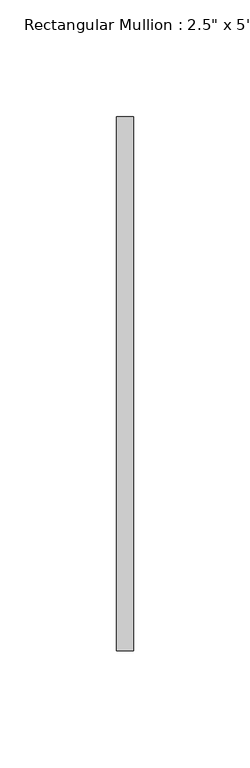
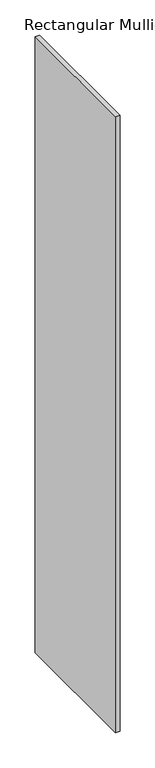
"""IFC4 building model written with IfcOpenShell, lengths in millimetres: member geometry."""

from ifc_helpers import new_model, si_unit, frame, origin, place, context, project, spatial, polyline, outline, extrude, source, transform, mapped, element, save


def member_f4ca0770(model_context):
    return source(origin(), model_context, "Body", "SweptSolid", [
        extrude(outline(polyline([(0.0, 114.3), (0.0, -114.3), (-7.239, -114.3), (-7.239, 114.3), (0.0, 114.3)])), frame((0.0, 0.0, -1066.8), z_axis=(0.0, 0.0, 1.0), x_axis=(1.0, 0.0, 0.0)), (0.0, 0.0, 1.0), 1066.8),
    ])


if __name__ == "__main__":
    model = new_model("IFC4")
    model_context = context("Model", 3, world=origin())
    ifc_project = project(units=[si_unit("LENGTHUNIT", "METRE", prefix="MILLI")], contexts=[model_context])
    site = spatial("IfcSite", under=ifc_project)
    building = spatial("IfcBuilding", under=site)
    placement = place(None, origin())
    member_shape = member_f4ca0770(model_context)
    element("IfcMember", 1, ObjectType="Rectangular Mullion : 2.5\" x 5\" rectangular", at=placement, inside=building, context=model_context, shape_type="MappedRepresentation", body=[
        mapped(member_shape, transform((0.0, 0.0, 0.0), x_axis=(1.0, 0.0, 0.0), y_axis=(0.0, 1.0, 0.0), z_axis=(0.0, 0.0, 1.0))),
    ])
    save(model, "model.ifc")

# Revit data of these elements
# Type "Rectangular Mullion : 2.5\" x 5\" rectangular"
#   built-in parameter 1007304 = 0.75 (stored number, unit not read)
#   built-in parameter 1007301 = 0.011875 (stored number, unit not read)
#   built-in parameter 1007300 = 0.011875 (stored number, unit not read)
# Element 1 (IfcMember, "Rectangular Mullion : 2.5\" x 5\" rectangular")
#   Materials on its faces: "WINDOW GLASS MATERIAL"
# Materials
#   "WINDOW GLASS MATERIAL": class "Generic", colour RGB 120 120 120, transparency 0, Cost = 0
